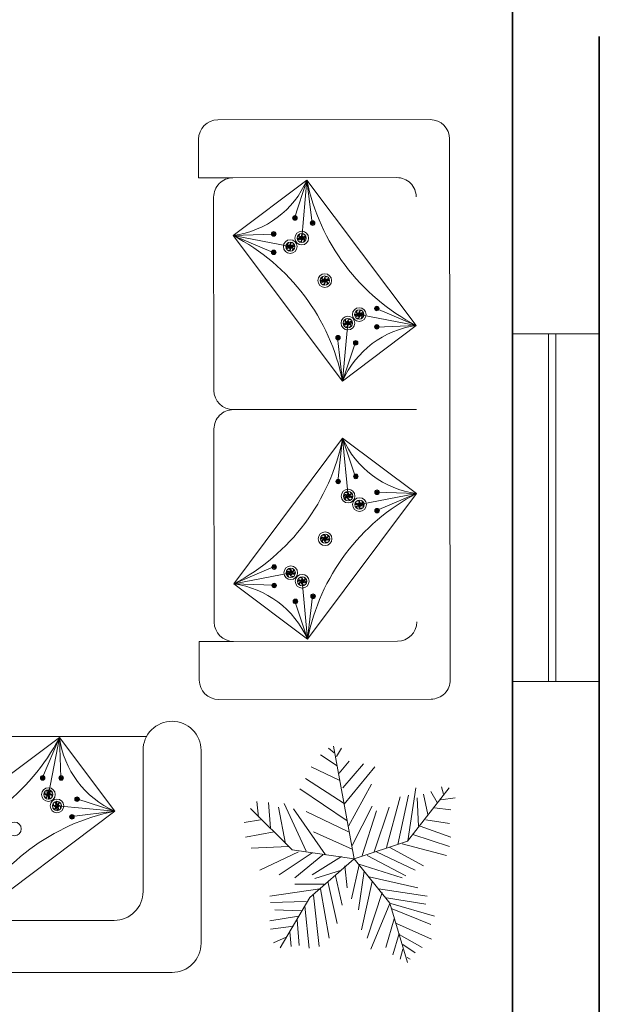
# Model space of a CAD drawing. Units: inches. Extents: x -61 to 1599, y -1316 to 257.
# Tile 178 of 204: x 1463 to 1523, y -937 to -835. Entities that reach past the tile are written whole.
import ezdxf

# ---------------------------------------------------------------- set-up
doc = ezdxf.new("R2010")
doc.units = ezdxf.units.IN
doc.header["$MEASUREMENT"] = 0
doc.layers.add('FUR', color=83, linetype='Continuous')
for name, color, linetype, lineweight in [('FURNITURE', 83, 'Continuous', 18), ('WALLS', 4, 'Continuous', 35), ('WINDOWS', 220, 'Continuous', 18)]:
    doc.layers.add(name, color=color, linetype=linetype, lineweight=lineweight)

# ---------------------------------------------------------------- blocks, each defined once
blk = doc.blocks.new('*U529')
at = {"layer": 'FUR'}
blk.add_open_spline([(0.01, 0.24), (-0.09, 0.14), (-0.29, -0.05), (0.22, -0.05), (0.07, -0.19), (0.01, -0.24)], degree=3, knots=[0, 0, 0, 0, 0.2846533, 0.5662105, 0.736751, 0.736751, 0.736751, 0.736751], dxfattribs=at)
blk = doc.blocks.new('*U530')
at = {"layer": 'FURNITURE', "transparency": 16777216}
for p, rotation in [((662.52, -238.49), 60), ((662.53, -238.73), 120), ((662.93, -238.46), 300), ((662.94, -238.7), 240), ((662.74, -238.83), 180)]:
    blk.add_blockref('*U529', p, dxfattribs=dict(at, rotation=rotation))
blk.add_blockref('*U529', (662.72, -238.36), dxfattribs=at)
blk = doc.blocks.new('*U543')
at = {"layer": 'FUR'}
blk.add_open_spline([(0.01, 0.24), (-0.09, 0.14), (-0.29, -0.05), (0.22, -0.05), (0.07, -0.19), (0.01, -0.24)], degree=3, knots=[0, 0, 0, 0, 0.2846533, 0.5662105, 0.736751, 0.736751, 0.736751, 0.736751], dxfattribs=at)
blk = doc.blocks.new('*U563')
at = {"layer": 'FURNITURE', "transparency": 16777216}
for p, rotation in [((662.52, -238.49), 60), ((662.53, -238.73), 120), ((662.93, -238.46), 300), ((662.94, -238.7), 240), ((662.74, -238.83), 180)]:
    blk.add_blockref('*U543', p, dxfattribs=dict(at, rotation=rotation))
blk.add_blockref('*U543', (662.72, -238.36), dxfattribs=at)
blk = doc.blocks.new('*U564')
at = {"layer": 'FUR'}
blk.add_open_spline([(0, 0.08), (-0.03, 0.05), (-0.1, -0.02), (0.08, -0.02), (0.02, -0.06), (0, -0.08)], degree=3, knots=[0, 0, 0, 0, 0.0954578, 0.1898773, 0.2470677, 0.2470677, 0.2470677, 0.2470677], dxfattribs=at)
blk = doc.blocks.new('*U565')
at = {"layer": 'FURNITURE', "transparency": 16777216}
for p, rotation in [((222.17, -79.98), 60), ((222.18, -80.06), 120), ((222.31, -79.97), 300), ((222.25, -80.09), 180), ((222.32, -80.05), 240)]:
    blk.add_blockref('*U564', p, dxfattribs=dict(at, rotation=rotation))
blk.add_blockref('*U564', (222.24, -79.93), dxfattribs=at)
blk = doc.blocks.new('*U531')
at = {"layer": 'FUR'}
blk.add_open_spline([(0, 0.08), (-0.03, 0.05), (-0.1, -0.02), (0.08, -0.02), (0.02, -0.06), (0, -0.08)], degree=3, knots=[0, 0, 0, 0, 0.0954578, 0.1898773, 0.2470677, 0.2470677, 0.2470677, 0.2470677], dxfattribs=at)
blk = doc.blocks.new('*U532')
at = {"layer": 'FURNITURE', "transparency": 16777216}
for p, rotation in [((222.17, -79.98), 60), ((222.18, -80.06), 120), ((222.31, -79.97), 300), ((222.25, -80.09), 180), ((222.32, -80.05), 240)]:
    blk.add_blockref('*U531', p, dxfattribs=dict(at, rotation=rotation))
blk.add_blockref('*U531', (222.24, -79.93), dxfattribs=at)
blk = doc.blocks.new('*U533')
at = {"layer": 'FUR'}
blk.add_open_spline([(0, 0.08), (-0.03, 0.05), (-0.1, -0.02), (0.08, -0.02), (0.02, -0.06), (0, -0.08)], degree=3, knots=[0, 0, 0, 0, 0.0954578, 0.1898773, 0.2470677, 0.2470677, 0.2470677, 0.2470677], dxfattribs=at)
blk = doc.blocks.new('*U534')
at = {"layer": 'FURNITURE', "transparency": 16777216}
for p, rotation in [((222.17, -79.98), 60), ((222.18, -80.06), 120), ((222.31, -79.97), 300), ((222.25, -80.09), 180), ((222.32, -80.05), 240)]:
    blk.add_blockref('*U533', p, dxfattribs=dict(at, rotation=rotation))
blk.add_blockref('*U533', (222.24, -79.93), dxfattribs=at)
blk = doc.blocks.new('*U535')
at = {"layer": 'FUR'}
blk.add_open_spline([(0, 0.08), (-0.03, 0.05), (-0.1, -0.02), (0.08, -0.02), (0.02, -0.06), (0, -0.08)], degree=3, knots=[0, 0, 0, 0, 0.0954578, 0.1898773, 0.2470677, 0.2470677, 0.2470677, 0.2470677], dxfattribs=at)
blk = doc.blocks.new('*U536')
at = {"layer": 'FURNITURE', "transparency": 16777216}
for p, rotation in [((222.17, -79.98), 60), ((222.18, -80.06), 120), ((222.31, -79.97), 300), ((222.25, -80.09), 180), ((222.32, -80.05), 240)]:
    blk.add_blockref('*U535', p, dxfattribs=dict(at, rotation=rotation))
blk.add_blockref('*U535', (222.24, -79.93), dxfattribs=at)
blk = doc.blocks.new('*U537')
at = {"layer": 'FUR'}
blk.add_open_spline([(0, 0.08), (-0.03, 0.05), (-0.1, -0.02), (0.08, -0.02), (0.02, -0.06), (0, -0.08)], degree=3, knots=[0, 0, 0, 0, 0.0954578, 0.1898773, 0.2470677, 0.2470677, 0.2470677, 0.2470677], dxfattribs=at)
blk = doc.blocks.new('*U538')
at = {"layer": 'FURNITURE', "transparency": 16777216}
for p, rotation in [((222.17, -79.98), 60), ((222.18, -80.06), 120), ((222.31, -79.97), 300), ((222.25, -80.09), 180), ((222.32, -80.05), 240)]:
    blk.add_blockref('*U537', p, dxfattribs=dict(at, rotation=rotation))
blk.add_blockref('*U537', (222.24, -79.93), dxfattribs=at)
blk = doc.blocks.new('*U539')
at = {"layer": 'FUR'}
blk.add_open_spline([(0, 0.08), (-0.03, 0.05), (-0.1, -0.02), (0.08, -0.02), (0.02, -0.06), (0, -0.08)], degree=3, knots=[0, 0, 0, 0, 0.0954578, 0.1898773, 0.2470677, 0.2470677, 0.2470677, 0.2470677], dxfattribs=at)
blk = doc.blocks.new('*U540')
at = {"layer": 'FURNITURE', "transparency": 16777216}
for p, rotation in [((222.17, -79.98), 60), ((222.18, -80.06), 120), ((222.31, -79.97), 300), ((222.25, -80.09), 180), ((222.32, -80.05), 240)]:
    blk.add_blockref('*U539', p, dxfattribs=dict(at, rotation=rotation))
blk.add_blockref('*U539', (222.24, -79.93), dxfattribs=at)
blk = doc.blocks.new('*U541')
at = {"layer": 'FUR'}
blk.add_open_spline([(0, 0.08), (-0.03, 0.05), (-0.1, -0.02), (0.08, -0.02), (0.02, -0.06), (0, -0.08)], degree=3, knots=[0, 0, 0, 0, 0.0954578, 0.1898773, 0.2470677, 0.2470677, 0.2470677, 0.2470677], dxfattribs=at)
blk = doc.blocks.new('*U567')
at = {"layer": 'FURNITURE', "transparency": 16777216}
for p, rotation in [((222.17, -79.98), 60), ((222.18, -80.06), 120), ((222.31, -79.97), 300), ((222.25, -80.09), 180), ((222.32, -80.05), 240)]:
    blk.add_blockref('*U541', p, dxfattribs=dict(at, rotation=rotation))
blk.add_blockref('*U541', (222.24, -79.93), dxfattribs=at)
blk = doc.blocks.new('*U568')
at = {"layer": 'FUR'}
blk.add_open_spline([(0, 0.08), (-0.03, 0.05), (-0.1, -0.02), (0.08, -0.02), (0.02, -0.06), (0, -0.08)], degree=3, knots=[0, 0, 0, 0, 0.0954578, 0.1898773, 0.2470677, 0.2470677, 0.2470677, 0.2470677], dxfattribs=at)
blk = doc.blocks.new('*U569')
at = {"layer": 'FURNITURE', "transparency": 16777216}
for p, rotation in [((222.17, -79.98), 60), ((222.18, -80.06), 120), ((222.31, -79.97), 300), ((222.25, -80.09), 180), ((222.32, -80.05), 240)]:
    blk.add_blockref('*U568', p, dxfattribs=dict(at, rotation=rotation))
blk.add_blockref('*U568', (222.24, -79.93), dxfattribs=at)
blk = doc.blocks.new('*U570')
at = {"layer": 'FUR'}
blk.add_open_spline([(0.01, 0.24), (-0.09, 0.14), (-0.29, -0.05), (0.22, -0.05), (0.07, -0.19), (0.01, -0.24)], degree=3, knots=[0, 0, 0, 0, 0.2846533, 0.5662105, 0.736751, 0.736751, 0.736751, 0.736751], dxfattribs=at)
blk = doc.blocks.new('*U571')
at = {"layer": 'FURNITURE', "transparency": 16777216}
for p, rotation in [((662.52, -238.49), 60), ((662.53, -238.73), 120), ((662.93, -238.46), 300), ((662.94, -238.7), 240), ((662.74, -238.83), 180)]:
    blk.add_blockref('*U570', p, dxfattribs=dict(at, rotation=rotation))
blk.add_blockref('*U570', (662.72, -238.36), dxfattribs=at)
blk = doc.blocks.new('*U572')
at = {"layer": 'FUR'}
blk.add_open_spline([(0.01, 0.24), (-0.09, 0.14), (-0.29, -0.05), (0.22, -0.05), (0.07, -0.19), (0.01, -0.24)], degree=3, knots=[0, 0, 0, 0, 0.2846533, 0.5662105, 0.736751, 0.736751, 0.736751, 0.736751], dxfattribs=at)
blk = doc.blocks.new('*U528')
at = {"layer": 'FURNITURE', "transparency": 16777216}
for p, rotation in [((662.52, -238.49), 60), ((662.53, -238.73), 120), ((662.93, -238.46), 300), ((662.94, -238.7), 240), ((662.74, -238.83), 180)]:
    blk.add_blockref('*U572', p, dxfattribs=dict(at, rotation=rotation))
blk.add_blockref('*U572', (662.72, -238.36), dxfattribs=at)
blk = doc.blocks.new('*U542')
at = {"layer": 'FUR'}
blk.add_open_spline([(0.01, 0.24), (-0.09, 0.14), (-0.29, -0.05), (0.22, -0.05), (0.07, -0.19), (0.01, -0.24)], degree=3, knots=[0, 0, 0, 0, 0.2846533, 0.5662105, 0.736751, 0.736751, 0.736751, 0.736751], dxfattribs=at)
blk = doc.blocks.new('*U566')
at = {"layer": 'FURNITURE', "transparency": 16777216}
for p, rotation in [((662.52, -238.49), 60), ((662.53, -238.73), 120), ((662.93, -238.46), 300), ((662.94, -238.7), 240), ((662.74, -238.83), 180)]:
    blk.add_blockref('*U542', p, dxfattribs=dict(at, rotation=rotation))
blk.add_blockref('*U542', (662.72, -238.36), dxfattribs=at)
blk = doc.blocks.new('*U525')
at = {"layer": 'FUR'}
blk.add_open_spline([(0.01, 0.24), (-0.09, 0.14), (-0.29, -0.05), (0.22, -0.05), (0.07, -0.19), (0.01, -0.24)], degree=3, knots=[0, 0, 0, 0, 0.2846533, 0.5662105, 0.736751, 0.736751, 0.736751, 0.736751], dxfattribs=at)
blk = doc.blocks.new('*U526')
at = {"layer": 'FURNITURE', "transparency": 16777216}
for p, rotation in [((662.52, -238.49), 60), ((662.53, -238.73), 120), ((662.93, -238.46), 300), ((662.94, -238.7), 240), ((662.74, -238.83), 180)]:
    blk.add_blockref('*U525', p, dxfattribs=dict(at, rotation=rotation))
blk.add_blockref('*U525', (662.72, -238.36), dxfattribs=at)
blk = doc.blocks.new('*U562')
at = {"layer": 'FUR'}
blk.add_open_spline([(0.01, 0.24), (-0.09, 0.14), (-0.29, -0.05), (0.22, -0.05), (0.07, -0.19), (0.01, -0.24)], degree=3, knots=[0, 0, 0, 0, 0.2846533, 0.5662105, 0.736751, 0.736751, 0.736751, 0.736751], dxfattribs=at)
blk = doc.blocks.new('*U544')
at = {"layer": 'FURNITURE', "transparency": 16777216}
for p, rotation in [((662.52, -238.49), 60), ((662.53, -238.73), 120), ((662.93, -238.46), 300), ((662.94, -238.7), 240), ((662.74, -238.83), 180)]:
    blk.add_blockref('*U562', p, dxfattribs=dict(at, rotation=rotation))
blk.add_blockref('*U562', (662.72, -238.36), dxfattribs=at)
blk = doc.blocks.new('*U545')
at = {"layer": 'FUR'}
blk.add_open_spline([(0, 0.08), (-0.03, 0.05), (-0.1, -0.02), (0.08, -0.02), (0.02, -0.06), (0, -0.08)], degree=3, knots=[0, 0, 0, 0, 0.0954578, 0.1898773, 0.2470677, 0.2470677, 0.2470677, 0.2470677], dxfattribs=at)
blk = doc.blocks.new('*U546')
at = {"layer": 'FURNITURE', "transparency": 16777216}
for p, rotation in [((222.17, -79.98), 60), ((222.18, -80.06), 120), ((222.31, -79.97), 300), ((222.25, -80.09), 180), ((222.32, -80.05), 240)]:
    blk.add_blockref('*U545', p, dxfattribs=dict(at, rotation=rotation))
blk.add_blockref('*U545', (222.24, -79.93), dxfattribs=at)
blk = doc.blocks.new('*U527')
at = {"layer": 'FUR'}
blk.add_open_spline([(0, 0.08), (-0.03, 0.05), (-0.1, -0.02), (0.08, -0.02), (0.02, -0.06), (0, -0.08)], degree=3, knots=[0, 0, 0, 0, 0.0954578, 0.1898773, 0.2470677, 0.2470677, 0.2470677, 0.2470677], dxfattribs=at)
blk = doc.blocks.new('*U551')
at = {"layer": 'FURNITURE', "transparency": 16777216}
for p, rotation in [((222.17, -79.98), 60), ((222.18, -80.06), 120), ((222.31, -79.97), 300), ((222.25, -80.09), 180), ((222.32, -80.05), 240)]:
    blk.add_blockref('*U527', p, dxfattribs=dict(at, rotation=rotation))
blk.add_blockref('*U527', (222.24, -79.93), dxfattribs=at)
blk = doc.blocks.new('*U552')
at = {"layer": 'FUR'}
blk.add_open_spline([(0, 0.08), (-0.03, 0.05), (-0.1, -0.02), (0.08, -0.02), (0.02, -0.06), (0, -0.08)], degree=3, knots=[0, 0, 0, 0, 0.0954578, 0.1898773, 0.2470677, 0.2470677, 0.2470677, 0.2470677], dxfattribs=at)
blk = doc.blocks.new('*U553')
at = {"layer": 'FURNITURE', "transparency": 16777216}
for p, rotation in [((222.17, -79.98), 60), ((222.18, -80.06), 120), ((222.31, -79.97), 300), ((222.25, -80.09), 180), ((222.32, -80.05), 240)]:
    blk.add_blockref('*U552', p, dxfattribs=dict(at, rotation=rotation))
blk.add_blockref('*U552', (222.24, -79.93), dxfattribs=at)
blk = doc.blocks.new('*U554')
at = {"layer": 'FUR'}
blk.add_open_spline([(0, 0.08), (-0.03, 0.05), (-0.1, -0.02), (0.08, -0.02), (0.02, -0.06), (0, -0.08)], degree=3, knots=[0, 0, 0, 0, 0.0954578, 0.1898773, 0.2470677, 0.2470677, 0.2470677, 0.2470677], dxfattribs=at)
blk = doc.blocks.new('*U555')
at = {"layer": 'FURNITURE', "transparency": 16777216}
for p, rotation in [((222.17, -79.98), 60), ((222.18, -80.06), 120), ((222.31, -79.97), 300), ((222.25, -80.09), 180), ((222.32, -80.05), 240)]:
    blk.add_blockref('*U554', p, dxfattribs=dict(at, rotation=rotation))
blk.add_blockref('*U554', (222.24, -79.93), dxfattribs=at)
blk = doc.blocks.new('*U556')
at = {"layer": 'FUR'}
blk.add_open_spline([(0, 0.08), (-0.03, 0.05), (-0.1, -0.02), (0.08, -0.02), (0.02, -0.06), (0, -0.08)], degree=3, knots=[0, 0, 0, 0, 0.0954578, 0.1898773, 0.2470677, 0.2470677, 0.2470677, 0.2470677], dxfattribs=at)
blk = doc.blocks.new('*U557')
at = {"layer": 'FURNITURE', "transparency": 16777216}
for p, rotation in [((222.17, -79.98), 60), ((222.18, -80.06), 120), ((222.31, -79.97), 300), ((222.25, -80.09), 180), ((222.32, -80.05), 240)]:
    blk.add_blockref('*U556', p, dxfattribs=dict(at, rotation=rotation))
blk.add_blockref('*U556', (222.24, -79.93), dxfattribs=at)
blk = doc.blocks.new('*U558')
at = {"layer": 'FUR'}
blk.add_open_spline([(0, 0.08), (-0.03, 0.05), (-0.1, -0.02), (0.08, -0.02), (0.02, -0.06), (0, -0.08)], degree=3, knots=[0, 0, 0, 0, 0.0954578, 0.1898773, 0.2470677, 0.2470677, 0.2470677, 0.2470677], dxfattribs=at)
blk = doc.blocks.new('*U559')
at = {"layer": 'FURNITURE', "transparency": 16777216}
for p, rotation in [((222.17, -79.98), 60), ((222.18, -80.06), 120), ((222.31, -79.97), 300), ((222.25, -80.09), 180), ((222.32, -80.05), 240)]:
    blk.add_blockref('*U558', p, dxfattribs=dict(at, rotation=rotation))
blk.add_blockref('*U558', (222.24, -79.93), dxfattribs=at)
blk = doc.blocks.new('*U560')
at = {"layer": 'FUR'}
blk.add_open_spline([(0, 0.08), (-0.03, 0.05), (-0.1, -0.02), (0.08, -0.02), (0.02, -0.06), (0, -0.08)], degree=3, knots=[0, 0, 0, 0, 0.0954578, 0.1898773, 0.2470677, 0.2470677, 0.2470677, 0.2470677], dxfattribs=at)
blk = doc.blocks.new('*U548')
at = {"layer": 'FURNITURE', "transparency": 16777216}
for p, rotation in [((222.17, -79.98), 60), ((222.18, -80.06), 120), ((222.31, -79.97), 300), ((222.25, -80.09), 180), ((222.32, -80.05), 240)]:
    blk.add_blockref('*U560', p, dxfattribs=dict(at, rotation=rotation))
blk.add_blockref('*U560', (222.24, -79.93), dxfattribs=at)
blk = doc.blocks.new('*U549')
at = {"layer": 'FUR'}
blk.add_open_spline([(0, 0.08), (-0.03, 0.05), (-0.1, -0.02), (0.08, -0.02), (0.02, -0.06), (0, -0.08)], degree=3, knots=[0, 0, 0, 0, 0.0954578, 0.1898773, 0.2470677, 0.2470677, 0.2470677, 0.2470677], dxfattribs=at)
blk = doc.blocks.new('*U550')
at = {"layer": 'FURNITURE', "transparency": 16777216}
for p, rotation in [((222.17, -79.98), 60), ((222.18, -80.06), 120), ((222.31, -79.97), 300), ((222.25, -80.09), 180), ((222.32, -80.05), 240)]:
    blk.add_blockref('*U549', p, dxfattribs=dict(at, rotation=rotation))
blk.add_blockref('*U549', (222.24, -79.93), dxfattribs=at)
blk = doc.blocks.new('*U521')
at = {"layer": 'FUR'}
blk.add_open_spline([(0.01, 0.24), (-0.09, 0.14), (-0.29, -0.05), (0.22, -0.05), (0.07, -0.19), (0.01, -0.24)], degree=3, knots=[0, 0, 0, 0, 0.2846533, 0.5662105, 0.736751, 0.736751, 0.736751, 0.736751], dxfattribs=at)
blk = doc.blocks.new('*U522')
at = {"layer": 'FURNITURE', "transparency": 16777216}
for p, rotation in [((662.52, -238.49), 60), ((662.53, -238.73), 120), ((662.93, -238.46), 300), ((662.94, -238.7), 240), ((662.74, -238.83), 180)]:
    blk.add_blockref('*U521', p, dxfattribs=dict(at, rotation=rotation))
blk.add_blockref('*U521', (662.72, -238.36), dxfattribs=at)
blk = doc.blocks.new('*U523')
at = {"layer": 'FUR'}
blk.add_open_spline([(0.01, 0.24), (-0.09, 0.14), (-0.29, -0.05), (0.22, -0.05), (0.07, -0.19), (0.01, -0.24)], degree=3, knots=[0, 0, 0, 0, 0.2846533, 0.5662105, 0.736751, 0.736751, 0.736751, 0.736751], dxfattribs=at)
blk = doc.blocks.new('*U524')
at = {"layer": 'FURNITURE', "transparency": 16777216}
for p, rotation in [((662.52, -238.49), 60), ((662.53, -238.73), 120), ((662.93, -238.46), 300), ((662.94, -238.7), 240), ((662.74, -238.83), 180)]:
    blk.add_blockref('*U523', p, dxfattribs=dict(at, rotation=rotation))
blk.add_blockref('*U523', (662.72, -238.36), dxfattribs=at)
blk = doc.blocks.new('*U561')
at = {"layer": 'FUR'}
blk.add_open_spline([(0.01, 0.24), (-0.09, 0.14), (-0.29, -0.05), (0.22, -0.05), (0.07, -0.19), (0.01, -0.24)], degree=3, knots=[0, 0, 0, 0, 0.2846533, 0.5662105, 0.736751, 0.736751, 0.736751, 0.736751], dxfattribs=at)
blk = doc.blocks.new('*U547')
at = {"layer": 'FURNITURE', "transparency": 16777216}
for p, rotation in [((662.52, -238.49), 60), ((662.53, -238.73), 120), ((662.93, -238.46), 300), ((662.94, -238.7), 240), ((662.74, -238.83), 180)]:
    blk.add_blockref('*U561', p, dxfattribs=dict(at, rotation=rotation))
blk.add_blockref('*U561', (662.72, -238.36), dxfattribs=at)
blk = doc.blocks.new('*U264')
for p, q in [((-10.186, 53.64), (-13.084, 55.962)), ((0, 0), (-10.5, 57)), ((-9.099, 51.782), (-6.563, 55.962)), ((-8.737, 47.138), (-17.069, 52.711)), ((-7.288, 39.707), (-21.778, 46.673)), ((-7.65, 43.423), (-2.578, 49.46)), ((-5.839, 35.992), (4.667, 48.067)), ((-5.114, 27.632), (10.463, 46.673)), ((-5.114, 28.097), (-24.676, 40.636)), ((-3.665, 19.273), (-27.574, 35.527)), ((-2.941, 16.486), (8.652, 37.85)), ((27, 9), (48, 36)), ((27.127, 9.056), (31.112, 35.992)), ((44.153, 36.456), (45.239, 32.741)), ((16.259, 5.805), (23.142, 31.348)), ((22.055, 7.198), (27.489, 32.277)), ((31.836, 30.883), (32.561, 16.486)), ((35.096, 32.741), (37.27, 22.524)), ((38.719, 34.134), (41.979, 28.561)), ((43.791, 29.954), (51.036, 30.883)), ((-31.5, 4.5), (-52.5, 25.5)), ((-48.585, 21.131), (-49.309, 29.026)), ((-43.513, 28.561), (-42.427, 15.558)), ((-38.442, 26.239), (-34.819, 7.663)), ((-35.544, 28.097), (-24.314, 3.947)), ((-14.533, 2.09), (-30.834, 25.31)), ((-1.129, 6.734), (9.014, 26.704)), ((10.101, 3.483), (17.708, 26.239)), ((40.53, 25.775), (48.862, 24.846)), ((-24.314, 23.917), (-2.941, 13.7)), ((3.942, 1.625), (11.187, 24.381)), ((-47.498, 19.737), (-55.83, 18.344)), ((33.285, 16.486), (48.862, 10.913)), ((36.183, 19.737), (48.137, 17.88)), ((-40.615, 13.7), (-55.105, 10.913)), ((-20.691, 13.7), (-1.129, 4.876)), ((29.662, 12.307), (48.137, 6.269)), ((-33.37, 6.269), (-52.207, 5.34)), ((0, 0), (27, 9)), ((18.07, 5.805), (35.096, -3.483)), ((24.229, 7.663), (46.688, 1.625)), ((-28.299, 3.483), (-47.86, -5.805)), ((-21.416, 3.018), (-38.079, -8.128)), ((0, 0), (-31.5, 4.5)), ((-15.982, 2.09), (-30.11, -9.521)), ((0, 0), (-22.5, -19.5)), ((-6.563, 1.161), (-21.416, -8.128)), ((0, 0), (18, -22.5)), ((6.478, 1.625), (26.04, -8.592)), ((11.187, 3.483), (30.749, -5.805)), ((-4.752, -3.483), (-3.665, -14.629)), ((2.493, -3.019), (-1.491, -20.202)), ((1.769, -2.555), (24.229, -9.521)), ((-6.563, -5.805), (-19.967, -9.985)), ((-9.461, -8.592), (-6.201, -23.453)), ((5.029, -6.27), (2.131, -25.775)), ((7.565, -9.056), (32.198, -14.629)), ((-15.257, -12.772), (-30.11, -12.772)), ((-13.446, -11.378), (-8.737, -32.741)), ((9.014, -11.378), (3.58, -35.992)), ((-17.431, -15.094), (-42.789, -18.809)), ((-22.5, -19.5), (-37.5, -45)), ((-20.691, -18.345), (-17.793, -44.352)), ((-17.069, -15.094), (-12.721, -40.172)), ((14.085, -16.951), (6.478, -40.172)), ((12.274, -15.094), (36.907, -18.809)), ((16.259, -19.738), (36.183, -22.989)), ((-24.314, -21.596), (-42.427, -22.06)), ((-25.038, -23.918), (-22.865, -45.281)), ((18.07, -22.524), (8.289, -45.745)), ((18, -22.5), (27, -52.5)), ((18.433, -22.524), (40.53, -29.026)), ((-28.299, -29.026), (-42.789, -31.348)), ((-26.849, -26.24), (-40.253, -25.775)), ((19.157, -25.311), (38.719, -33.206)), ((-30.834, -34.135), (-42.427, -35.528)), ((-29.023, -30.884), (-27.936, -43.887)), ((20.244, -30.419), (15.897, -44.816)), ((21.331, -32.741), (39.081, -40.636)), ((-34.457, -39.708), (-40.978, -42.494)), ((-32.646, -36.921), (-31.921, -44.352)), ((22.78, -37.85), (19.519, -48.532)), ((22.78, -38.314), (34.372, -44.816)), ((24.591, -43.423), (30.749, -47.603)), ((24.591, -45.745), (23.142, -50.854)), ((26.764, -49.925), (28.213, -50.854))]:
    blk.add_line(p, q)
blk = doc.blocks.new('WIN-36IN')
for p, q in [((0, 4.5), (0, 9)), ((0, 9), (0, 0)), ((36, 9), (36, 0)), ((0, 5.26), (36, 5.26)), ((0, 4.5), (36, 4.5)), ((0, 4.5), (36, 4.5))]:
    blk.add_line(p, q)
blk = doc.blocks.new('*U348')
at = {"layer": 'FUR'}
blk.add_open_spline([(0, 0.08), (-0.03, 0.05), (-0.1, -0.02), (0.08, -0.02), (0.02, -0.06), (0, -0.08)], degree=3, knots=[0, 0, 0, 0, 0.0954578, 0.1898773, 0.2470677, 0.2470677, 0.2470677, 0.2470677], dxfattribs=at)
blk = doc.blocks.new('*U349')
at = {"layer": 'FUR', "transparency": 16777216}
for p, rotation in [((222.17, -79.98), 60), ((222.18, -80.06), 120), ((222.31, -79.97), 300), ((222.25, -80.09), 180), ((222.32, -80.05), 240)]:
    blk.add_blockref('*U348', p, dxfattribs=dict(at, rotation=rotation))
blk.add_blockref('*U348', (222.24, -79.93), dxfattribs=at)
blk = doc.blocks.new('*U356')
at = {"layer": 'FUR'}
blk.add_open_spline([(0.01, 0.24), (-0.09, 0.14), (-0.29, -0.05), (0.22, -0.05), (0.07, -0.19), (0.01, -0.24)], degree=3, knots=[0, 0, 0, 0, 0.2846533, 0.5662105, 0.736751, 0.736751, 0.736751, 0.736751], dxfattribs=at)
blk = doc.blocks.new('*U357')
at = {"layer": 'FUR', "transparency": 16777216}
for p, rotation in [((662.52, -238.49), 60), ((662.53, -238.73), 120), ((662.93, -238.46), 300), ((662.94, -238.7), 240), ((662.74, -238.83), 180)]:
    blk.add_blockref('*U356', p, dxfattribs=dict(at, rotation=rotation))
blk.add_blockref('*U356', (662.72, -238.36), dxfattribs=at)
blk = doc.blocks.new('*U340')
at = {"layer": 'FUR'}
blk.add_open_spline([(0.01, 0.24), (-0.09, 0.14), (-0.29, -0.05), (0.22, -0.05), (0.07, -0.19), (0.01, -0.24)], degree=3, knots=[0, 0, 0, 0, 0.2846533, 0.5662105, 0.736751, 0.736751, 0.736751, 0.736751], dxfattribs=at)
blk = doc.blocks.new('*U341')
at = {"layer": 'FUR', "transparency": 16777216}
for p, rotation in [((662.52, -238.49), 60), ((662.53, -238.73), 120), ((662.93, -238.46), 300), ((662.94, -238.7), 240), ((662.74, -238.83), 180)]:
    blk.add_blockref('*U340', p, dxfattribs=dict(at, rotation=rotation))
blk.add_blockref('*U340', (662.72, -238.36), dxfattribs=at)
blk = doc.blocks.new('*U346')
at = {"layer": 'FUR'}
blk.add_open_spline([(0, 0.08), (-0.03, 0.05), (-0.1, -0.02), (0.08, -0.02), (0.02, -0.06), (0, -0.08)], degree=3, knots=[0, 0, 0, 0, 0.0954578, 0.1898773, 0.2470677, 0.2470677, 0.2470677, 0.2470677], dxfattribs=at)
blk = doc.blocks.new('*U347')
at = {"layer": 'FUR', "transparency": 16777216}
for p, rotation in [((222.17, -79.98), 60), ((222.18, -80.06), 120), ((222.31, -79.97), 300), ((222.25, -80.09), 180), ((222.32, -80.05), 240)]:
    blk.add_blockref('*U346', p, dxfattribs=dict(at, rotation=rotation))
blk.add_blockref('*U346', (222.24, -79.93), dxfattribs=at)
blk = doc.blocks.new('*U354')
at = {"layer": 'FUR'}
blk.add_open_spline([(0, 0.08), (-0.03, 0.05), (-0.1, -0.02), (0.08, -0.02), (0.02, -0.06), (0, -0.08)], degree=3, knots=[0, 0, 0, 0, 0.0954578, 0.1898773, 0.2470677, 0.2470677, 0.2470677, 0.2470677], dxfattribs=at)
blk = doc.blocks.new('*U355')
at = {"layer": 'FUR', "transparency": 16777216}
for p, rotation in [((222.17, -79.98), 60), ((222.18, -80.06), 120), ((222.31, -79.97), 300), ((222.25, -80.09), 180), ((222.32, -80.05), 240)]:
    blk.add_blockref('*U354', p, dxfattribs=dict(at, rotation=rotation))
blk.add_blockref('*U354', (222.24, -79.93), dxfattribs=at)
blk = doc.blocks.new('*U350')
at = {"layer": 'FUR'}
blk.add_open_spline([(0, 0.08), (-0.03, 0.05), (-0.1, -0.02), (0.08, -0.02), (0.02, -0.06), (0, -0.08)], degree=3, knots=[0, 0, 0, 0, 0.0954578, 0.1898773, 0.2470677, 0.2470677, 0.2470677, 0.2470677], dxfattribs=at)
blk = doc.blocks.new('*U342')
at = {"layer": 'FUR', "transparency": 16777216}
for p, rotation in [((222.17, -79.98), 60), ((222.18, -80.06), 120), ((222.31, -79.97), 300), ((222.25, -80.09), 180), ((222.32, -80.05), 240)]:
    blk.add_blockref('*U350', p, dxfattribs=dict(at, rotation=rotation))
blk.add_blockref('*U350', (222.24, -79.93), dxfattribs=at)
blk = doc.blocks.new('SOFA-THREE-SEAT-ALT')
for p, q in [((78.37, 24.44), (57, 24.44)), ((69.34, 24.33), (67.59, 20.19)), ((69.34, 24.33), (68.19, 18.42)), ((69.34, 24.33), (69.49, 20.19)), ((67.6, 20.14), (67.6, 20.3)), ((67.6, 20.14), (67.6, 19.98)), ((69.51, 20.14), (69.51, 20.3)), ((69.51, 20.14), (69.51, 19.98)), ((68.19, 18.42), (68.19, 18.9)), ((68.19, 18.42), (68.19, 17.95)), ((69.08, 17.24), (69.08, 17.72)), ((75.07, 16.69), (71.14, 17.99)), ((71.16, 17.94), (71.16, 18.1)), ((71.16, 17.94), (71.16, 17.78)), ((75.07, 16.69), (69.08, 17.24)), ((69.08, 17.24), (69.08, 16.77)), ((75.07, 16.69), (70.61, 16.16)), ((70.63, 16.11), (70.63, 16.27)), ((70.63, 16.11), (70.63, 15.95))]:
    blk.add_line(p, q)
blk.add_lwpolyline([(78, 8.38), (78, 23, -0.414214), (81, 26), (81, 26, -0.414214), (84, 23), (84, 3, -0.414214), (81, 0), (3, 0, -0.414214), (0, 3), (0, 23, -0.414214), (3, 26), (3, 26, -0.414214), (6, 23), (6, 8.38, 0.414214), (9, 5.38), (75, 5.38, 0.414214)], format="xyb", close=True)
blk.add_lwpolyline([(54.27, 13.03), (69.34, 24.33), (75.07, 16.69), (60.01, 5.38)], close=True)
for centre, radius in [((67.6, 20.14), 0.238), ((67.6, 20.14), 0.16), ((69.51, 20.14), 0.238), ((69.51, 20.14), 0.16), ((68.19, 18.42), 0.71), ((68.19, 18.42), 0.476), ((69.08, 17.24), 0.71), ((69.08, 17.24), 0.476), ((71.16, 17.94), 0.238), ((71.16, 17.94), 0.16), ((70.63, 16.11), 0.238), ((64.67, 14.86), 0.71), ((70.63, 16.11), 0.16)]:
    blk.add_circle(centre, radius)
for centre, radius, start, end in [((50.05, 34.34), 21.73, 281.2044, 332.5684), ((79.06, 25.66), 9.82, 187.747, 246.0258), ((79.3, -4.63), 21.73, 101.2044, 152.5684)]:
    blk.add_arc(centre, radius, start, end)
at = {"rotation": 180}
for name, p in [('*U349', (289.85, -59.87)), ('*U347', (291.75, -59.87)), ('*U357', (730.92, -220.17)), ('*U341', (731.81, -221.35)), ('*U342', (293.4, -62.07)), ('*U355', (292.87, -63.9))]:
    blk.add_blockref(name, p, dxfattribs=at)

msp = doc.modelspace()

# ---------------------------------------------------------------- linework, layer by layer
at = {"layer": 'FURNITURE'}
for p, q in [((1484.7579, -851.661), (1481.1999, -851.6658)), ((1484.7579, -851.661), (1501.7299, -851.6376)), ((1492.4247, -851.8992), (1491.1247, -855.8346)), ((1492.4247, -851.8992), (1491.8773, -857.894)), ((1492.4247, -851.8992), (1492.9538, -856.3642)), ((1482.7607, -853.6637), (1482.7882, -873.6637)), ((1491.1772, -855.8152), (1491.0174, -855.8154)), ((1491.1772, -855.8152), (1491.337, -855.815)), ((1493.0062, -856.3448), (1492.8464, -856.345)), ((1493.0062, -856.3448), (1493.166, -856.3445)), ((1484.7866, -857.6476), (1488.9281, -857.4878)), ((1484.7866, -857.6476), (1490.6987, -858.781)), ((1484.7866, -857.6476), (1488.9307, -859.392)), ((1488.9805, -857.4684), (1488.8207, -857.4686)), ((1488.9805, -857.4684), (1489.1403, -857.4682)), ((1491.8773, -857.894), (1491.4008, -857.8946)), ((1491.8773, -857.894), (1492.3538, -857.8933)), ((1488.9831, -859.3725), (1488.8233, -859.3727)), ((1488.9831, -859.3725), (1489.1429, -859.3723)), ((1490.6987, -858.781), (1490.2222, -858.7817)), ((1490.6987, -858.781), (1491.1752, -858.7803)), ((1494.2688, -862.2981), (1493.7923, -862.2988)), ((1494.2688, -862.2981), (1494.7452, -862.2975)), ((1499.6593, -865.1849), (1499.4995, -865.1851)), ((1503.7509, -866.9486), (1499.6068, -865.2043)), ((1499.6593, -865.1849), (1499.8191, -865.1847)), ((1497.8388, -865.8152), (1497.3623, -865.8159)), ((1497.8388, -865.8152), (1498.3153, -865.8146)), ((1503.7509, -866.9486), (1497.8388, -865.8152)), ((1496.1128, -872.6971), (1496.6602, -866.7023)), ((1496.6602, -866.7023), (1496.1837, -866.7029)), ((1496.6602, -866.7023), (1497.1367, -866.7016)), ((1499.6619, -867.089), (1499.5021, -867.0892)), ((1503.7509, -866.9486), (1499.6094, -867.1084)), ((1499.6619, -867.089), (1499.8217, -867.0888)), ((1495.6362, -868.2126), (1495.4764, -868.2129)), ((1496.1128, -872.6971), (1495.5838, -868.2321)), ((1495.6362, -868.2126), (1495.796, -868.2124)), ((1496.1128, -872.6971), (1497.4128, -868.7616)), ((1497.4652, -868.7422), (1497.3054, -868.7424)), ((1497.4652, -868.7422), (1497.625, -868.742)), ((1484.7909, -875.661), (1503.7629, -875.6349)), ((1484.7909, -875.661), (1484.7909, -875.661)), ((1482.8212, -897.6637), (1482.7937, -877.6637)), ((1496.121, -878.6194), (1495.6042, -883.0858)), ((1496.121, -878.6194), (1496.6848, -884.6127)), ((1496.121, -878.6194), (1497.4317, -882.5512)), ((1497.4842, -882.5705), (1497.3244, -882.5707)), ((1497.4842, -882.5705), (1497.644, -882.5703)), ((1495.6567, -883.1051), (1495.4969, -883.1053)), ((1495.6567, -883.1051), (1495.8165, -883.1049)), ((1496.6848, -884.6127), (1496.2084, -884.6133)), ((1496.6848, -884.6127), (1497.1613, -884.612)), ((1503.7748, -884.3468), (1497.8659, -885.4964)), ((1499.6854, -884.2177), (1499.5256, -884.2179)), ((1503.7748, -884.3468), (1499.6329, -884.1984)), ((1503.7748, -884.3468), (1499.6355, -886.1025)), ((1499.6854, -884.2177), (1499.8452, -884.2175)), ((1497.8659, -885.4964), (1497.3894, -885.4971)), ((1497.8659, -885.4964), (1498.3424, -885.4958)), ((1499.688, -886.1218), (1499.5283, -886.122)), ((1499.688, -886.1218), (1499.8478, -886.1216)), ((1494.3055, -889.0234), (1493.829, -889.024)), ((1494.3055, -889.0234), (1494.782, -889.0227)), ((1484.8361, -893.6999), (1488.9754, -891.9442)), ((1489.0279, -891.9635), (1488.8681, -891.9637)), ((1489.0279, -891.9635), (1489.1877, -891.9633)), ((1484.8361, -893.6999), (1490.7451, -892.5503)), ((1490.7451, -892.5503), (1490.2686, -892.5509)), ((1490.7451, -892.5503), (1491.2216, -892.5496)), ((1484.8361, -893.6999), (1488.978, -893.8483)), ((1489.0305, -893.8676), (1488.8708, -893.8678)), ((1489.0305, -893.8676), (1489.1903, -893.8674)), ((1491.9261, -893.4341), (1491.4496, -893.4347)), ((1491.9261, -893.4341), (1492.4026, -893.4334)), ((1492.49, -899.4273), (1491.9261, -893.4341)), ((1492.49, -899.4273), (1493.0068, -894.9609)), ((1493.0593, -894.9802), (1492.8995, -894.9804)), ((1493.0593, -894.9802), (1493.2191, -894.9799)), ((1491.2318, -895.5148), (1491.072, -895.515)), ((1492.49, -899.4273), (1491.1793, -895.4955)), ((1491.2318, -895.5148), (1491.3915, -895.5146)), ((1484.8239, -899.6609), (1481.2659, -899.6658)), ((1484.8239, -899.6609), (1501.7958, -899.6376))]:
    msp.add_line(p, q, dxfattribs=at)
msp.add_lwpolyline([(1481.2659, -899.6658), (1481.2714, -903.6658, 0.41421356), (1483.2742, -905.6631), (1505.2741, -905.6328, 0.41421369), (1507.2714, -903.6301), (1507.1944, -847.6301, 0.41421343), (1505.1916, -845.6329), (1483.1917, -845.6631, 0.41421356), (1481.1944, -847.6658), (1481.1999, -851.6658)], format="xyb", dxfattribs=at)
for points in [[(1496.1128, -872.6971), (1484.7866, -857.6476), (1492.4247, -851.8992), (1503.7509, -866.9486)], [(1496.121, -878.6194), (1484.8361, -893.6999), (1492.49, -899.4273), (1503.7748, -884.3468)]]:
    msp.add_lwpolyline(points, close=True, dxfattribs=at)
for centre, radius in [((1491.1772, -855.8152), 0.2382), ((1491.1772, -855.8152), 0.1598), ((1493.0062, -856.3448), 0.2382), ((1493.0062, -856.3448), 0.1598), ((1488.9805, -857.4684), 0.2382), ((1488.9805, -857.4684), 0.1598), ((1491.8773, -857.894), 0.7104), ((1490.6987, -858.781), 0.7104), ((1490.6987, -858.781), 0.4765), ((1491.8773, -857.894), 0.4765), ((1488.9831, -859.3725), 0.2382), ((1488.9831, -859.3725), 0.1598), ((1494.2688, -862.2981), 0.7104), ((1494.2688, -862.2981), 0.4765), ((1497.8388, -865.8152), 0.7104), ((1497.8388, -865.8152), 0.4765), ((1499.6593, -865.1849), 0.2382), ((1499.6593, -865.1849), 0.1598), ((1496.6602, -866.7023), 0.7104), ((1496.6602, -866.7023), 0.4765), ((1499.6619, -867.089), 0.2382), ((1499.6619, -867.089), 0.1598), ((1495.6362, -868.2126), 0.2382), ((1495.6362, -868.2126), 0.1598), ((1497.4652, -868.7422), 0.2382), ((1497.4652, -868.7422), 0.1598), ((1497.4842, -882.5705), 0.2382), ((1497.4842, -882.5705), 0.1598), ((1495.6567, -883.1051), 0.2382), ((1495.6567, -883.1051), 0.1598), ((1496.6848, -884.6127), 0.7104), ((1496.6848, -884.6127), 0.4765), ((1497.8659, -885.4964), 0.7104), ((1499.6854, -884.2177), 0.2382), ((1499.6854, -884.2177), 0.1598), ((1497.8659, -885.4964), 0.4765), ((1499.688, -886.1218), 0.2382), ((1499.688, -886.1218), 0.1598), ((1494.3055, -889.0234), 0.7104), ((1494.3055, -889.0234), 0.4765), ((1489.0279, -891.9635), 0.2382), ((1489.0279, -891.9635), 0.1598), ((1490.7451, -892.5503), 0.7104), ((1490.7451, -892.5503), 0.4765), ((1491.9261, -893.4341), 0.7104), ((1491.9261, -893.4341), 0.4765), ((1489.0305, -893.8676), 0.2382), ((1489.0305, -893.8676), 0.1598), ((1493.0593, -894.9802), 0.2382), ((1493.0593, -894.9802), 0.1598), ((1491.2318, -895.5148), 0.2382), ((1491.2318, -895.5148), 0.1598)]:
    msp.add_circle(centre, radius, dxfattribs=at)
for centre, radius, start, end in [((1484.7607, -853.661), 2, 90.078764, 180.078764), ((1483.45, -847.923), 9.816, 277.825767, 336.104516), ((1513.7357, -847.6473), 21.731, 191.283178, 242.647105), ((1501.7326, -853.6376), 2, 0.078749, 90.078764), ((1474.8019, -876.9489), 21.731, 11.283178, 62.647105), ((1505.0875, -876.6732), 9.816, 97.825767, 156.104516), ((1484.7882, -873.661), 2, 180.078764, 270.078764), ((1484.7937, -877.661), 2, 90.078764, 180.078764), ((1474.7984, -874.4261), 21.731, 297.510392, 348.87432), ((1505.0847, -874.6186), 9.816, 204.052981, 262.33173), ((1513.8126, -903.6206), 21.731, 117.510392, 168.87432), ((1483.5263, -903.4282), 9.816, 24.052981, 82.33173), ((1484.8212, -897.6609), 2, 180.078764, 270.078764), ((1501.7931, -897.6376), 2, 270.078764, 0.078749)]:
    msp.add_arc(centre, radius, start, end, dxfattribs=at)
at = {"layer": 'WALLS'}
for p, q in [((1513.7028, -783.169), (1513.7028, -945.169)), ((1522.7028, -1211.169), (1522.7028, -837.0151))]:
    msp.add_line(p, q, dxfattribs=at)

# ---------------------------------------------------------------- block references
at = {"layer": 'FURNITURE'}
for name, p, rotation in [('*U548', (1570.884, -633.4605), 270.0787336990067), ('*U550', (1572.713, -633.9901), 270.0787336990067), ('*U557', (1568.6874, -635.1137), 270.0787336990067), ('*U522', (1728.383, -195.7236), 270.0787336990067), ('*U547', (1729.5615, -194.8366), 270.0787336990067), ('*U559', (1568.69, -637.0178), 270.0787336990067), ('*U526', (1731.953, -199.2408), 270.0787336990067), ('*U544', (1735.5231, -202.7579), 270.0787336990067), ('*U546', (1579.3661, -642.8302), 270.0787336990067), ('*U524', (1734.3445, -203.6449), 270.0787336990067), ('*U551', (1579.3687, -644.7343), 270.0787336990067), ('*U555', (1575.343, -645.8579), 270.0787336990067), ('*U553', (1577.1721, -646.3875), 270.0787336990067), ('SOFA-THREE-SEAT-ALT', (1397.4562, -933.9417), 0.0082401218147832)]:
    msp.add_blockref(name, p, dxfattribs=dict(at, rotation=rotation))
at = {"layer": 'FURNITURE', "xscale": -1, "rotation": 270.0787636990076}
for name, p in [('*U534', (1577.802, -1104.7052)), ('*U536', (1575.9744, -1105.2399)), ('*U528', (1736.1909, -1547.0142)), ('*U532', (1580.0032, -1106.3524)), ('*U563', (1737.3719, -1547.8979)), ('*U565', (1580.0058, -1108.2566)), ('*U530', (1733.8115, -1551.4249)), ('*U540', (1569.3457, -1114.0982)), ('*U571', (1730.2511, -1554.9518)), ('*U566', (1731.4321, -1555.8356)), ('*U538', (1569.3483, -1116.0024)), ('*U569', (1573.3771, -1117.1149)), ('*U567', (1571.5495, -1117.6495))]:
    msp.add_blockref(name, p, dxfattribs=at)
at = {"layer": 'FURNITURE', "xscale": 0.2045054661246738, "yscale": 0.2045054661246738, "zscale": 0.2045054661246738}
msp.add_blockref('*U264', (1497.3277, -922.1728), dxfattribs=at)
at = {"layer": 'WINDOWS', "rotation": 89.99999999999984}
msp.add_blockref('WIN-36IN', (1522.7029, -903.8181), dxfattribs=at)

doc.saveas('drawing.dxf')
